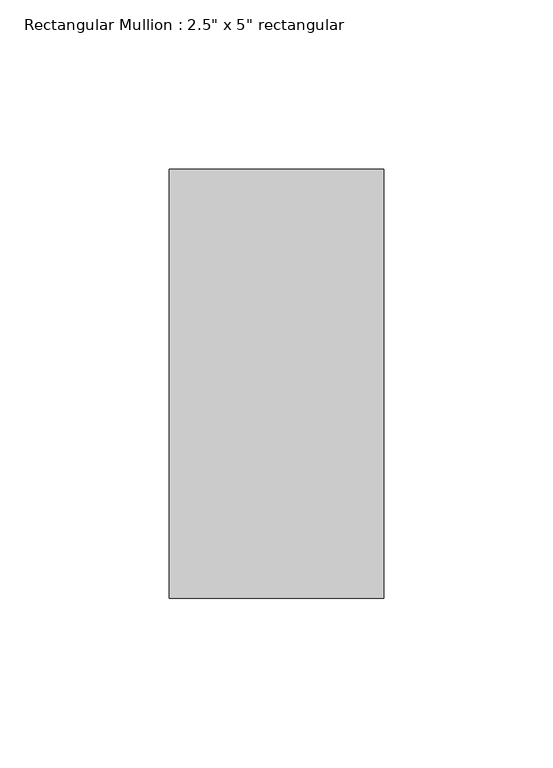
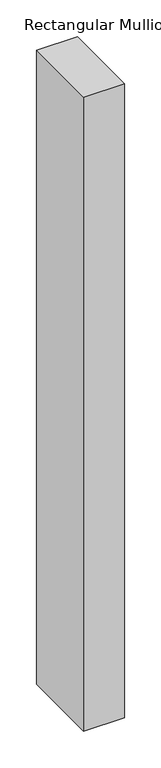
"""IFC4 building model written with IfcOpenShell, lengths in millimetres: member geometry."""

from ifc_helpers import new_model, si_unit, frame, origin, place, context, project, spatial, polyline, outline, extrude, source, transform, mapped, element, save


def member_501daf10(model_context):
    return source(origin(), model_context, "Body", "SweptSolid", [
        extrude(outline(polyline([(31.75, 63.5), (31.75, -63.5), (-31.75, -63.5), (-31.75, 63.5), (31.75, 63.5)])), frame((0.0, 0.0, -1047.3490947), z_axis=(0.0, 0.0, 1.0), x_axis=(1.0, 0.0, 0.0)), (0.0, 0.0, 1.0), 1047.3490947),
    ])


if __name__ == "__main__":
    model = new_model("IFC4")
    model_context = context("Model", 3, world=origin())
    ifc_project = project(units=[si_unit("LENGTHUNIT", "METRE", prefix="MILLI")], contexts=[model_context])
    site = spatial("IfcSite", under=ifc_project)
    building = spatial("IfcBuilding", under=site)
    placement = place(None, origin())
    member_shape = member_501daf10(model_context)
    element("IfcMember", 1, ObjectType="Rectangular Mullion : 2.5\" x 5\" rectangular", at=placement, inside=building, context=model_context, shape_type="MappedRepresentation", body=[
        mapped(member_shape, transform((0.0, 0.0, 0.0), x_axis=(1.0, 0.0, 0.0), y_axis=(0.0, 1.0, 0.0), z_axis=(0.0, 0.0, 1.0))),
    ])
    save(model, "model.ifc")

# Revit data of these elements
# Type "Rectangular Mullion : 2.5\" x 5\" rectangular"
#   built-in parameter 1007304 = 0.416667 (stored number, unit not read)
#   built-in parameter 1007301 = 0.104167 (stored number, unit not read)
#   built-in parameter 1007300 = 0.104167 (stored number, unit not read)
# Element 1 (IfcMember, "Rectangular Mullion : 2.5\" x 5\" rectangular")
#   Materials on its faces: "Aluminum"
# Materials
#   "Aluminum": class "Metal", colour RGB 247 247 247, transparency 0, Description = "Aluminum 6061", Cost = 0
